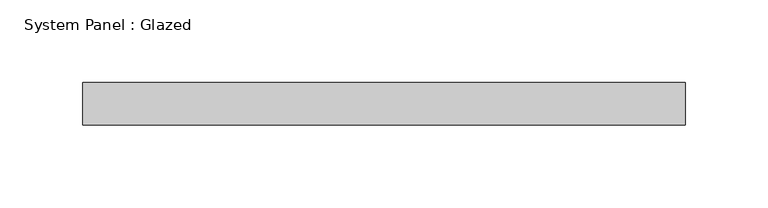
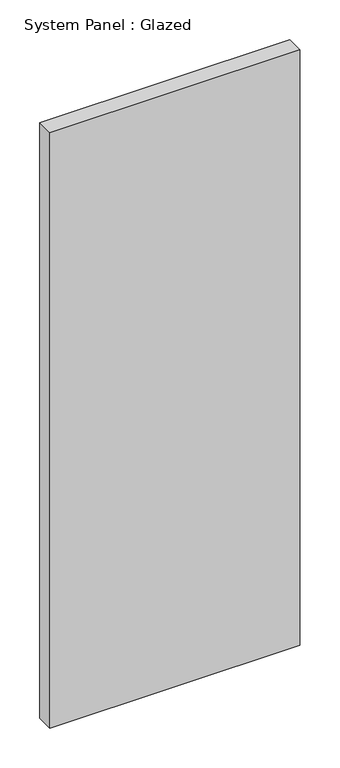
"""IFC4 building model written with IfcOpenShell, lengths in millimetres: plate geometry, System Panel : Glazed."""

from ifc_helpers import new_model, si_unit, origin, origin_with_axes, place, context, project, spatial, polyline, outline, extrude, source, transform, mapped, element, save


def system_panel_glazed_f2dc5d49(model_context):
    return source(origin(), model_context, "Body", "SweptSolid", [
        extrude(outline(polyline([(181.501417, 19.05), (-181.501417, 19.05), (-181.501417, 44.45), (181.501417, 44.45), (181.501417, 19.05)])), origin_with_axes(), (0.0, 0.0, 1.0), 914.4),
    ])


if __name__ == "__main__":
    model = new_model("IFC4")
    model_context = context("Model", 3, world=origin())
    ifc_project = project(units=[si_unit("LENGTHUNIT", "METRE", prefix="MILLI")], contexts=[model_context])
    site = spatial("IfcSite", under=ifc_project)
    building = spatial("IfcBuilding", under=site)
    placement = place(None, origin())
    system_panel_glazed_shape = system_panel_glazed_f2dc5d49(model_context)
    element("IfcPlate", 1, ObjectType="System Panel : Glazed", at=placement, inside=building, context=model_context, shape_type="MappedRepresentation", body=[
        mapped(system_panel_glazed_shape, transform((0.0, 0.0, 0.0), x_axis=(1.0, 0.0, 0.0), y_axis=(0.0, 1.0, 0.0), z_axis=(0.0, 0.0, 1.0))),
    ])
    save(model, "model.ifc")

# Revit data of these elements
# Type "System Panel : Glazed"
#   Construction Type Id = "GSP4R"
#   Analytic Construction = "1/8 in Pilkington single glazing"
#   Visual Light Transmittance = 0.9
#   Solar Heat Gain Coefficient = 0.86
#   Heat Transfer Coefficient (U) = 1.18115 BTU/(h·ft²·°F)
# Element 1 (IfcPlate, "System Panel : Glazed")
#   Materials on its faces: "Glass"
# Materials
#   "Glass": class "Glass", colour RGB 0 128 192, transparency 0.75, Description = "Soda Lime Glass", Cost = 0
